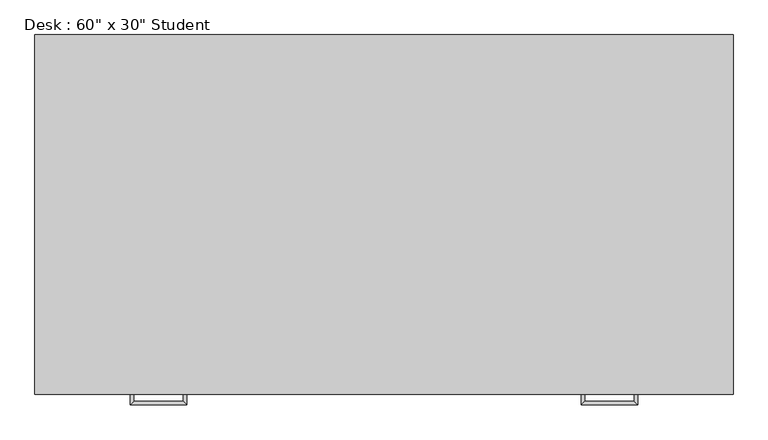
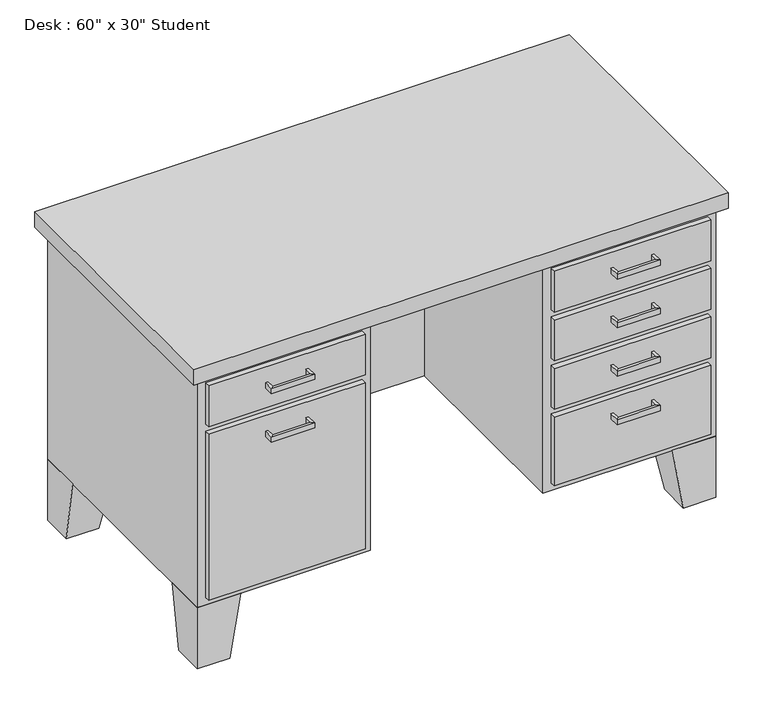
"""IFC4 building model written with IfcOpenShell, lengths in millimetres: furniture geometry."""

from ifc_helpers import new_model, si_unit, frame, origin, place, context, project, spatial, polyline, outline, extrude, faceted_brep, source, transform, mapped, element, save


def furniture_e086674a(model_context):
    return source(origin(), model_context, "Body", "SolidModel", [
        extrude(outline(polyline([(171.45, 76.2), (539.75, 76.2), (539.75, 63.5), (171.45, 63.5), (171.45, 76.2)])), frame((0.0, 0.0, 603.25), z_axis=(0.0, 0.0, 1.0), x_axis=(1.0, 0.0, 0.0)), (0.0, 0.0, 1.0), 101.6),
        extrude(outline(polyline([(171.45, 76.2), (539.75, 76.2), (539.75, 63.5), (171.45, 63.5), (171.45, 76.2)])), frame((0.0, 0.0, 171.45), z_axis=(0.0, 0.0, 1.0), x_axis=(1.0, 0.0, 0.0)), (0.0, 0.0, 1.0), 412.75),
        extrude(outline(polyline([(984.25, 76.2), (1352.55, 76.2), (1352.55, 63.5), (984.25, 63.5), (984.25, 76.2)])), frame((0.0, 0.0, 603.25), z_axis=(0.0, 0.0, 1.0), x_axis=(1.0, 0.0, 0.0)), (0.0, 0.0, 1.0), 101.6),
        extrude(outline(polyline([(984.25, 76.2), (1352.55, 76.2), (1352.55, 63.5), (984.25, 63.5), (984.25, 76.2)])), frame((0.0, 0.0, 171.45), z_axis=(0.0, 0.0, 1.0), x_axis=(1.0, 0.0, 0.0)), (0.0, 0.0, 1.0), 171.45),
        extrude(outline(polyline([(984.25, 76.2), (1352.55, 76.2), (1352.55, 63.5), (984.25, 63.5), (984.25, 76.2)])), frame((0.0, 0.0, 482.6), z_axis=(0.0, 0.0, 1.0), x_axis=(1.0, 0.0, 0.0)), (0.0, 0.0, 1.0), 101.6),
        extrude(outline(polyline([(984.25, 76.2), (1352.55, 76.2), (1352.55, 63.5), (984.25, 63.5), (984.25, 76.2)])), frame((0.0, 0.0, 361.95), z_axis=(0.0, 0.0, 1.0), x_axis=(1.0, 0.0, 0.0)), (0.0, 0.0, 1.0), 101.6),
        faceted_brep([(254.0, 76.2, 152.4), (254.0, 177.8, 152.4), (152.4, 177.8, 152.4), (152.4, 76.2, 152.4), (228.6, 76.2, 0.0), (152.4, 76.2, 0.0), (152.4, 152.4, 0.0), (228.6, 152.4, 0.0)], [[[0, 1, 2, 3]], [[4, 5, 6, 7]], [[4, 7, 1, 0]], [[7, 6, 2, 1]], [[6, 5, 3, 2]], [[5, 4, 0, 3]]]),
        faceted_brep([(254.0, 685.8, 152.4), (152.4, 685.8, 152.4), (152.4, 584.2, 152.4), (254.0, 584.2, 152.4), (228.6, 685.8, 0.0), (228.6, 609.6, 0.0), (152.4, 609.6, 0.0), (152.4, 685.8, 0.0)], [[[0, 1, 2, 3]], [[4, 5, 6, 7]], [[4, 7, 1, 0]], [[7, 6, 2, 1]], [[6, 5, 3, 2]], [[5, 4, 0, 3]]]),
        faceted_brep([(1270.0, 685.8, 152.4), (1270.0, 584.2, 152.4), (1371.6, 584.2, 152.4), (1371.6, 685.8, 152.4), (1295.4, 685.8, 0.0), (1371.6, 685.8, 0.0), (1371.6, 609.6, 0.0), (1295.4, 609.6, 0.0)], [[[0, 1, 2, 3]], [[4, 5, 6, 7]], [[4, 7, 1, 0]], [[7, 6, 2, 1]], [[6, 5, 3, 2]], [[5, 4, 0, 3]]]),
        faceted_brep([(1270.0, 76.2, 152.4), (1371.6, 76.2, 152.4), (1371.6, 177.8, 152.4), (1270.0, 177.8, 152.4), (1295.4, 76.2, 0.0), (1295.4, 152.4, 0.0), (1371.6, 152.4, 0.0), (1371.6, 76.2, 0.0)], [[[0, 1, 2, 3]], [[4, 5, 6, 7]], [[4, 7, 1, 0]], [[7, 6, 2, 1]], [[6, 5, 3, 2]], [[5, 4, 0, 3]]]),
        extrude(outline(polyline([(133.35, 57.15), (133.35, 704.85), (1390.65, 704.85), (1390.65, 57.15), (133.35, 57.15)])), frame((0.0, 0.0, 723.9), z_axis=(0.0, 0.0, 1.0), x_axis=(1.0, 0.0, 0.0)), (0.0, 0.0, 1.0), 38.1),
        extrude(outline(polyline([(965.2, 76.2), (965.2, 558.8), (558.8, 558.8), (558.8, 76.2), (152.4, 76.2), (152.4, 685.8), (1371.6, 685.8), (1371.6, 76.2), (965.2, 76.2)])), frame((0.0, 0.0, 152.4), z_axis=(0.0, 0.0, 1.0), x_axis=(1.0, 0.0, 0.0)), (0.0, 0.0, 1.0), 571.5),
        faceted_brep([(311.15, 63.5, 546.1), (311.15, 63.5, 533.4), (304.8, 63.5, 533.4), (304.8, 63.5, 546.1), (311.15, 44.45, 546.1), (311.15, 44.45, 533.4), (304.8, 38.1, 533.4), (304.8, 38.1, 546.1), (400.05, 44.45, 546.1), (400.05, 44.45, 533.4), (406.4, 38.1, 533.4), (406.4, 38.1, 546.1), (400.05, 63.5, 546.1), (406.4, 63.5, 546.1), (406.4, 63.5, 533.4), (400.05, 63.5, 533.4)], [[[0, 1, 2, 3]], [[1, 0, 4, 5]], [[2, 1, 5, 6]], [[3, 2, 6, 7]], [[0, 3, 7, 4]], [[5, 4, 8, 9]], [[6, 5, 9, 10]], [[7, 6, 10, 11]], [[4, 7, 11, 8]], [[12, 13, 14, 15]], [[9, 8, 12, 15]], [[10, 9, 15, 14]], [[11, 10, 14, 13]], [[8, 11, 13, 12]]]),
        faceted_brep([(311.15, 63.5, 666.75), (311.15, 63.5, 654.05), (304.8, 63.5, 654.05), (304.8, 63.5, 666.75), (311.15, 44.45, 666.75), (311.15, 44.45, 654.05), (304.8, 38.1, 654.05), (304.8, 38.1, 666.75), (400.05, 44.45, 666.75), (400.05, 44.45, 654.05), (406.4, 38.1, 654.05), (406.4, 38.1, 666.75), (400.05, 63.5, 666.75), (406.4, 63.5, 666.75), (406.4, 63.5, 654.05), (400.05, 63.5, 654.05)], [[[0, 1, 2, 3]], [[1, 0, 4, 5]], [[2, 1, 5, 6]], [[3, 2, 6, 7]], [[0, 3, 7, 4]], [[5, 4, 8, 9]], [[6, 5, 9, 10]], [[7, 6, 10, 11]], [[4, 7, 11, 8]], [[12, 13, 14, 15]], [[9, 8, 12, 15]], [[10, 9, 15, 14]], [[11, 10, 14, 13]], [[8, 11, 13, 12]]]),
        faceted_brep([(1212.85, 63.5, 304.8), (1219.2, 63.5, 304.8), (1219.2, 63.5, 292.1), (1212.85, 63.5, 292.1), (1212.85, 44.45, 304.8), (1219.2, 38.1, 304.8), (1219.2, 38.1, 292.1), (1212.85, 44.45, 292.1), (1123.95, 44.45, 304.8), (1117.6, 38.1, 304.8), (1117.6, 38.1, 292.1), (1123.95, 44.45, 292.1), (1123.95, 63.5, 304.8), (1123.95, 63.5, 292.1), (1117.6, 63.5, 292.1), (1117.6, 63.5, 304.8)], [[[0, 1, 2, 3]], [[1, 0, 4, 5]], [[2, 1, 5, 6]], [[3, 2, 6, 7]], [[0, 3, 7, 4]], [[5, 4, 8, 9]], [[6, 5, 9, 10]], [[7, 6, 10, 11]], [[4, 7, 11, 8]], [[12, 13, 14, 15]], [[9, 8, 12, 15]], [[10, 9, 15, 14]], [[11, 10, 14, 13]], [[8, 11, 13, 12]]]),
        faceted_brep([(1212.85, 63.5, 425.45), (1219.2, 63.5, 425.45), (1219.2, 63.5, 412.75), (1212.85, 63.5, 412.75), (1212.85, 44.45, 425.45), (1219.2, 38.1, 425.45), (1219.2, 38.1, 412.75), (1212.85, 44.45, 412.75), (1123.95, 44.45, 425.45), (1117.6, 38.1, 425.45), (1117.6, 38.1, 412.75), (1123.95, 44.45, 412.75), (1123.95, 63.5, 425.45), (1123.95, 63.5, 412.75), (1117.6, 63.5, 412.75), (1117.6, 63.5, 425.45)], [[[0, 1, 2, 3]], [[1, 0, 4, 5]], [[2, 1, 5, 6]], [[3, 2, 6, 7]], [[0, 3, 7, 4]], [[5, 4, 8, 9]], [[6, 5, 9, 10]], [[7, 6, 10, 11]], [[4, 7, 11, 8]], [[12, 13, 14, 15]], [[9, 8, 12, 15]], [[10, 9, 15, 14]], [[11, 10, 14, 13]], [[8, 11, 13, 12]]]),
        faceted_brep([(1212.85, 63.5, 546.1), (1219.2, 63.5, 546.1), (1219.2, 63.5, 533.4), (1212.85, 63.5, 533.4), (1212.85, 44.45, 546.1), (1219.2, 38.1, 546.1), (1219.2, 38.1, 533.4), (1212.85, 44.45, 533.4), (1123.95, 44.45, 546.1), (1117.6, 38.1, 546.1), (1117.6, 38.1, 533.4), (1123.95, 44.45, 533.4), (1123.95, 63.5, 546.1), (1123.95, 63.5, 533.4), (1117.6, 63.5, 533.4), (1117.6, 63.5, 546.1)], [[[0, 1, 2, 3]], [[1, 0, 4, 5]], [[2, 1, 5, 6]], [[3, 2, 6, 7]], [[0, 3, 7, 4]], [[5, 4, 8, 9]], [[6, 5, 9, 10]], [[7, 6, 10, 11]], [[4, 7, 11, 8]], [[12, 13, 14, 15]], [[9, 8, 12, 15]], [[10, 9, 15, 14]], [[11, 10, 14, 13]], [[8, 11, 13, 12]]]),
        faceted_brep([(1212.85, 63.5, 666.75), (1219.2, 63.5, 666.75), (1219.2, 63.5, 654.05), (1212.85, 63.5, 654.05), (1212.85, 44.45, 666.75), (1219.2, 38.1, 666.75), (1219.2, 38.1, 654.05), (1212.85, 44.45, 654.05), (1123.95, 44.45, 666.75), (1117.6, 38.1, 666.75), (1117.6, 38.1, 654.05), (1123.95, 44.45, 654.05), (1123.95, 63.5, 666.75), (1123.95, 63.5, 654.05), (1117.6, 63.5, 654.05), (1117.6, 63.5, 666.75)], [[[0, 1, 2, 3]], [[1, 0, 4, 5]], [[2, 1, 5, 6]], [[3, 2, 6, 7]], [[0, 3, 7, 4]], [[5, 4, 8, 9]], [[6, 5, 9, 10]], [[7, 6, 10, 11]], [[4, 7, 11, 8]], [[12, 13, 14, 15]], [[9, 8, 12, 15]], [[10, 9, 15, 14]], [[11, 10, 14, 13]], [[8, 11, 13, 12]]]),
    ])


if __name__ == "__main__":
    model = new_model("IFC4")
    model_context = context("Model", 3, world=origin())
    ifc_project = project(units=[si_unit("LENGTHUNIT", "METRE", prefix="MILLI")], contexts=[model_context])
    site = spatial("IfcSite", under=ifc_project)
    building = spatial("IfcBuilding", under=site)
    placement = place(None, origin())
    furniture_shape = furniture_e086674a(model_context)
    element("IfcFurniture", 1, ObjectType="Desk : 60\" x 30\" Student", at=placement, inside=building, context=model_context, shape_type="MappedRepresentation", body=[
        mapped(furniture_shape, transform((0.0, 0.0, 0.0), x_axis=(1.0, 0.0, 0.0), y_axis=(0.0, 1.0, 0.0), z_axis=(0.0, 0.0, 1.0))),
    ])
    save(model, "model.ifc")

# Revit data of these elements
# Type "Desk : 60\" x 30\" Student"
#   Assembly Code = "E2020200"
#   Depth = 2' - 0"
#   Height = 2' - 6"
#   Leg Height = 0' - 6"
#   Width = 4' - 0"
#   Body Material = Laminate, Ivory, Matte
#   Handle/Leg Material = Steel, Chrome Plated
#   Top Material = Cherry
#   Default Elevation = 0
# Element 1 (IfcFurniture, "Desk : 60\" x 30\" Student")
#   Materials on its faces: "Steel, Chrome Plated", "Laminate, Ivory, Matte", "Cherry"
# Materials
#   "Laminate, Ivory, Matte": class "Plastic", colour RGB 247 247 239, transparency 0, Description = "Plastic Laminate - Ivory, Matte", Cost = 0
#   "Steel, Chrome Plated": class "Metal", colour RGB 17 17 17, transparency 0, Description = "Chromiuim plated steel", Cost = 0
#   "Cherry": class "Wood", colour RGB 226 177 128, transparency 0, Description = "Prunus Serotina", Cost = 0
